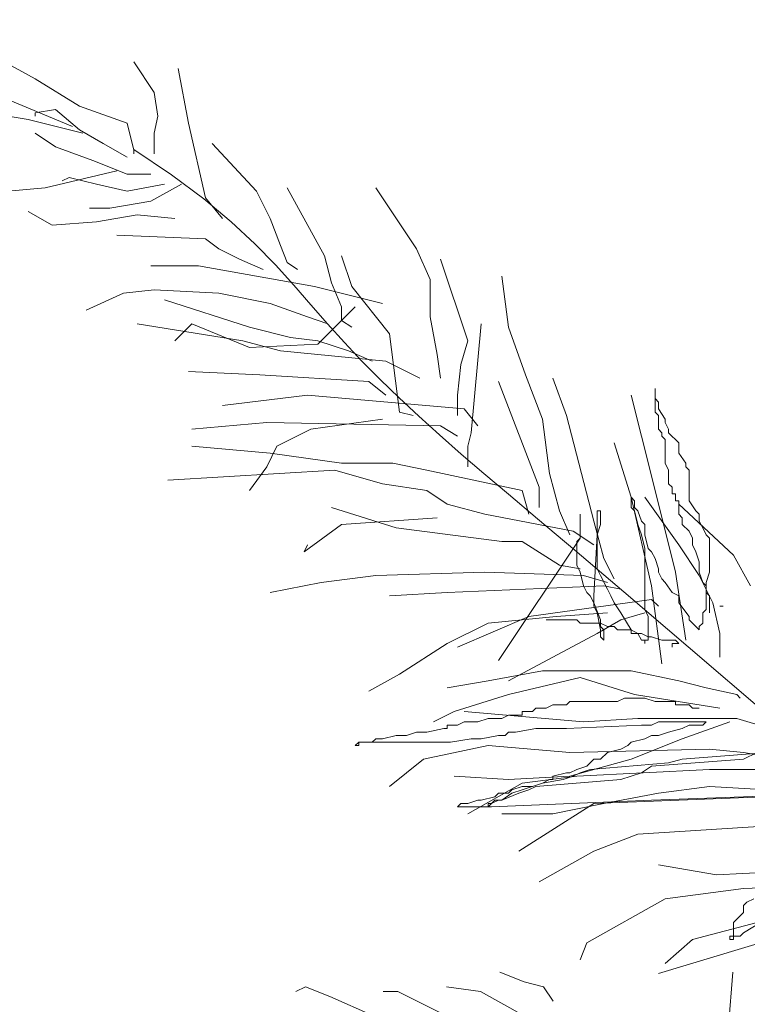
# Model space of a CAD drawing. Units: millimetres. Extents: x 595116 to 630915, y 909473 to 920225.
# Tile 36 of 134: x 629660.182 to 629665.643, y 919173.119 to 919180.516. Entities that reach past the tile are written whole.
import ezdxf

# ---------------------------------------------------------------- set-up
doc = ezdxf.new("R2010")
doc.units = ezdxf.units.MM
doc.layers.add('Dimension', color=3, linetype='Continuous', lineweight=18)
doc.layers.add('L-PLNT', color=85, linetype='Continuous', lineweight=13)
doc.styles.get("Standard").update_dxf_attribs({"font": 'arial.ttf'})
doc.dimstyles.new('ISO-25', dxfattribs={"dimtxt": 9, "dimasz": 6, "dimexe": 1.25, "dimexo": 0.625, "dimtad": 1, "dimlunit": 4, "dimtxsty": 'Standard', "dimcen": 2.5, "dimadec": 0, "dimazin": 0, "dimtfac": 1, "dimtmove": 0, "dimatfit": 3, "dimfxl": 1, "dimarcsym": 0})

# ---------------------------------------------------------------- blocks, each defined once
blk = doc.blocks.new('A$C4FB75ABC')
for p, q in [((0.4999, 4.2779), (0.7111, 4.1621)), ((0.9087, 4.1962), (0.9496, 4.1349)), ((0.9973, 4.1826), (1.0177, 4.0736)), ((0.7111, 4.1621), (0.7997, 4.1076)), ((0.7861, 4.0668), (0.6226, 4.1349)), ((0.9496, 4.1349), (0.9564, 4.0872)), ((0.752, 4.1008), (0.7111, 4.094)), ((0.7997, 4.06), (0.752, 4.1008)), ((0.7997, 4.1076), (0.8951, 4.0736)), ((0.6975, 4.0804), (0.6158, 4.094)), ((0.8065, 4.0532), (0.6975, 4.0804)), ((0.7111, 4.094), (0.7111, 4.0872)), ((0.9564, 4.0872), (0.9496, 4.0532)), ((0.8474, 4.0327), (0.7997, 4.06)), ((0.8951, 4.0736), (0.9087, 4.0191)), ((1.0177, 4.0736), (1.0518, 3.9238)), ((0.7111, 4.0532), (0.752, 4.0259)), ((0.9496, 4.0532), (0.9496, 4.0123)), ((0.752, 4.0259), (0.827, 3.9987)), ((0.8951, 4.0055), (0.8474, 4.0327)), ((0.9842, 3.9699), (0.9085, 4.0207)), ((1.0654, 4.0327), (1.154, 3.9374)), ((0.9087, 4.0191), (0.9087, 4.0123)), ((0.827, 3.9987), (0.8951, 3.9715)), ((0.8746, 3.9783), (0.7316, 3.9442)), ((0.7793, 3.9647), (0.7656, 3.9578)), ((0.8338, 3.951), (0.7793, 3.9647)), ((0.8951, 3.9715), (0.9428, 3.9715)), ((1.0487, 3.9217), (0.9842, 3.9699)), ((0.7316, 3.9442), (0.6566, 3.9374)), ((0.8951, 3.9374), (0.8338, 3.951)), ((0.97, 3.951), (0.8951, 3.9374)), ((1.0041, 3.951), (0.9428, 3.917)), ((1.2153, 3.9442), (1.2902, 3.808)), ((1.3924, 3.9442), (1.4742, 3.8217)), ((1.0518, 3.9238), (1.0858, 3.8829)), ((1.154, 3.9374), (1.1812, 3.8829)), ((0.861, 3.9034), (0.8201, 3.9034)), ((0.9428, 3.917), (0.861, 3.9034)), ((1.1035, 3.8758), (1.0487, 3.9217)), ((0.7452, 3.8693), (0.6975, 3.8966)), ((0.9155, 3.8897), (0.8338, 3.8761)), ((0.9905, 3.8829), (0.9155, 3.8897)), ((1.1812, 3.8829), (1.2017, 3.8285)), ((0.8338, 3.8761), (0.7452, 3.8693)), ((1.1506, 3.8319), (1.1035, 3.8758)), ((0.8746, 3.8489), (1.0518, 3.8421)), ((1.0518, 3.8421), (1.079, 3.8217)), ((1.1917, 3.7897), (1.1506, 3.8319)), ((1.2017, 3.8285), (1.2153, 3.7944)), ((1.079, 3.8217), (1.1199, 3.8012)), ((1.2902, 3.808), (1.3039, 3.7536)), ((1.3243, 3.808), (1.3447, 3.7467)), ((1.4742, 3.8217), (1.5014, 3.7604)), ((0.9428, 3.7876), (1.0382, 3.7876)), ((1.0382, 3.7876), (1.2698, 3.7467)), ((1.1199, 3.8012), (1.1676, 3.7808)), ((1.2284, 3.7492), (1.1917, 3.7897)), ((1.2153, 3.7944), (1.2357, 3.7808)), ((1.5219, 3.8012), (1.5764, 3.6378)), ((1.6445, 3.7672), (1.6581, 3.665)), ((1.2625, 3.7099), (1.2284, 3.7492)), ((1.2698, 3.7467), (1.4061, 3.7127)), ((1.3039, 3.7536), (1.3243, 3.7059)), ((1.3447, 3.7467), (1.4197, 3.6514)), ((1.5014, 3.7604), (1.5014, 3.6855)), ((0.8133, 3.6991), (0.8883, 3.7331)), ((0.8883, 3.7331), (0.9496, 3.7399)), ((0.9496, 3.7399), (1.079, 3.7331)), ((1.079, 3.7331), (1.1812, 3.7127)), ((0.97, 3.7195), (1.1403, 3.665)), ((1.1812, 3.7127), (1.2562, 3.6855)), ((1.2959, 3.6716), (1.2625, 3.7099)), ((1.3515, 3.7059), (1.2766, 3.631)), ((1.3243, 3.7059), (1.3243, 3.6787)), ((1.2562, 3.6855), (1.297, 3.6718)), ((1.5014, 3.6855), (1.5151, 3.6106)), ((0.9155, 3.6718), (1.1267, 3.6378)), ((1.0245, 3.6718), (0.9905, 3.6378)), ((1.1403, 3.6242), (1.0245, 3.6718)), ((1.3299, 3.6341), (1.2959, 3.6716)), ((1.3243, 3.6787), (1.3447, 3.665)), ((1.6036, 3.6718), (1.5832, 3.4539)), ((1.1403, 3.665), (1.2221, 3.6446)), ((1.4197, 3.6514), (1.4401, 3.4948)), ((1.6581, 3.665), (1.6922, 3.5697)), ((1.1267, 3.6378), (1.2017, 3.6174)), ((1.2766, 3.631), (1.1403, 3.6242)), ((1.2221, 3.6446), (1.2766, 3.6378)), ((1.2766, 3.6378), (1.3379, 3.6174)), ((1.365, 3.5971), (1.3299, 3.6341)), ((1.5764, 3.6378), (1.5627, 3.5901)), ((1.2017, 3.6174), (1.4129, 3.5969)), ((1.3379, 3.6174), (1.3856, 3.5969)), ((1.5151, 3.6106), (1.5219, 3.5629)), ((1.4014, 3.5604), (1.365, 3.5971)), ((1.4129, 3.5969), (1.481, 3.5629)), ((1.5627, 3.5901), (1.5559, 3.5288)), ((1.0177, 3.5765), (1.1608, 3.5697)), ((1.1608, 3.5697), (1.3788, 3.5561)), ((1.6922, 3.5697), (1.7263, 3.4812)), ((1.3788, 3.5561), (1.4129, 3.5288)), ((1.4393, 3.5237), (1.4014, 3.5604)), ((1.6377, 3.5561), (1.7194, 3.345)), ((1.7467, 3.5629), (1.7739, 3.488)), ((1.0858, 3.5084), (1.2562, 3.5288)), ((1.2562, 3.5288), (1.5696, 3.5016)), ((1.5559, 3.5288), (1.5559, 3.488)), ((1.9034, 3.5288), (1.9238, 3.4471)), ((1.9511, 3.4948), (1.9511, 3.5425)), ((1.9511, 3.5425), (1.9511, 3.522)), ((1.4788, 3.4868), (1.4393, 3.5237)), ((1.9511, 3.522), (1.9579, 3.5152)), ((1.9579, 3.5152), (1.9579, 3.5016)), ((1.4401, 3.4948), (1.4674, 3.488)), ((1.5696, 3.5016), (1.5968, 3.4676)), ((1.9579, 3.488), (1.9511, 3.4948)), ((1.9579, 3.5016), (1.9715, 3.4812)), ((1.0245, 3.4608), (1.1744, 3.4744)), ((1.1744, 3.4744), (1.5219, 3.4676)), ((1.4061, 3.4812), (1.263, 3.4608)), ((1.5201, 3.4494), (1.4788, 3.4868)), ((1.7263, 3.4812), (1.7399, 3.3722)), ((1.7739, 3.488), (1.8285, 3.2769)), ((1.9579, 3.4608), (1.9579, 3.488)), ((1.9715, 3.4812), (1.9715, 3.4744)), ((1.9715, 3.4744), (1.9783, 3.4608)), ((1.263, 3.4608), (1.1949, 3.4267)), ((1.5633, 3.4112), (1.5201, 3.4494)), ((1.5219, 3.4676), (1.5559, 3.4471)), ((1.5832, 3.4539), (1.5764, 3.4267)), ((1.9647, 3.4539), (1.9579, 3.4608)), ((1.9647, 3.4471), (1.9647, 3.4539)), ((1.9783, 3.4608), (1.9783, 3.4539)), ((1.9783, 3.4539), (1.9988, 3.4335)), ((1.8693, 3.4335), (1.9034, 3.3246)), ((1.9238, 3.4471), (1.9511, 3.3382)), ((1.9715, 3.4403), (1.9647, 3.4471)), ((1.9715, 3.3927), (1.9715, 3.4403)), ((1.9988, 3.4335), (1.9988, 3.4131)), ((1.0245, 3.4267), (1.1812, 3.4131)), ((1.1949, 3.4267), (1.1744, 3.3858)), ((1.1812, 3.4131), (1.3243, 3.3927)), ((1.6088, 3.3721), (1.5633, 3.4112)), ((1.5764, 3.4267), (1.5764, 3.3858)), ((1.9988, 3.4131), (2.0124, 3.3927)), ((1.3243, 3.3927), (1.4265, 3.3927)), ((1.4265, 3.3927), (1.4946, 3.379)), ((1.9783, 3.379), (1.9715, 3.3927)), ((2.0124, 3.3927), (2.0124, 3.3858)), ((0.9768, 3.3586), (1.3107, 3.379)), ((1.1744, 3.3858), (1.1403, 3.3382)), ((1.3107, 3.379), (1.4061, 3.3518)), ((1.4946, 3.379), (1.6854, 3.3382)), ((1.6577, 3.3307), (1.6088, 3.3721)), ((1.7399, 3.3722), (1.7603, 3.2973)), ((1.9783, 3.3518), (1.9783, 3.379)), ((2.0124, 3.3858), (2.0192, 3.379)), ((2.0192, 3.379), (2.0192, 3.3178)), ((1.4061, 3.3518), (1.4946, 3.3382)), ((1.9851, 3.345), (1.9783, 3.3518)), ((1.4946, 3.3382), (1.5355, 3.3109)), ((1.7159, 3.2817), (1.6577, 3.3307)), ((1.6854, 3.3382), (1.699, 3.2905)), ((1.7194, 3.345), (1.7194, 3.3041)), ((1.9511, 3.3382), (1.992, 3.1748)), ((1.9851, 3.3314), (1.9851, 3.345)), ((1.992, 3.3314), (1.9851, 3.3314)), ((1.992, 3.3178), (1.992, 3.3314)), ((1.5355, 3.3109), (1.6104, 3.2905)), ((1.9102, 3.3178), (1.9034, 3.3246)), ((1.9034, 3.3246), (1.9034, 3.3041)), ((1.9034, 3.3246), (1.9443, 3.1475)), ((1.9102, 3.3041), (1.9102, 3.3178)), ((1.9306, 3.3246), (1.9988, 3.2292)), ((1.9988, 3.3178), (1.992, 3.3178)), ((1.9988, 3.2905), (1.9988, 3.3178)), ((1.9988, 3.3109), (2.1078, 3.2088)), ((2.0192, 3.3178), (2.0328, 3.2973)), ((1.3039, 3.3041), (1.4333, 3.2633)), ((1.7603, 3.2973), (1.7808, 3.2497)), ((1.8421, 3.2973), (1.8353, 3.2973)), ((1.8353, 3.2973), (1.8353, 3.2497)), ((1.8421, 3.2701), (1.8421, 3.2973)), ((1.9034, 3.3041), (1.9102, 3.2973)), ((1.917, 3.2973), (1.9102, 3.3041)), ((1.9102, 3.2973), (1.917, 3.2701)), ((1.9238, 3.2769), (1.917, 3.2973)), ((2.0328, 3.2973), (2.0396, 3.2905)), ((1.5151, 3.2837), (1.3243, 3.2701)), ((1.6104, 3.2905), (1.7876, 3.2565)), ((1.7906, 3.2188), (1.7159, 3.2817)), ((1.8012, 3.2429), (1.8012, 3.2905)), ((1.8012, 3.2905), (1.8012, 3.2429)), ((1.8285, 3.2769), (1.8489, 3.202)), ((1.9306, 3.2701), (1.9238, 3.2769)), ((2.0056, 3.2837), (1.9988, 3.2905)), ((2.0056, 3.2701), (2.0056, 3.2837)), ((2.0396, 3.2905), (2.0396, 3.2769)), ((2.0396, 3.2769), (2.0465, 3.2633)), ((1.3243, 3.2701), (1.2494, 3.2156)), ((1.4333, 3.2633), (1.6445, 3.236)), ((1.7876, 3.2565), (1.8285, 3.2292)), ((1.8353, 3.2497), (1.8421, 3.2701)), ((1.917, 3.2701), (1.9238, 3.2497)), ((1.9306, 3.2497), (1.9306, 3.2701)), ((2.0192, 3.2565), (2.0056, 3.2701)), ((2.026, 3.2429), (2.0192, 3.2565)), ((2.0465, 3.2633), (2.0533, 3.2497)), ((1.8012, 3.2429), (1.6377, 2.9977)), ((1.6445, 3.236), (1.6854, 3.236)), ((1.6854, 3.236), (1.7603, 3.1884)), ((1.7944, 3.236), (1.8012, 3.2429)), ((1.7944, 3.1884), (1.7944, 3.236)), ((1.8353, 3.2497), (1.8285, 3.1271)), ((1.8353, 3.1816), (1.8353, 3.2497)), ((1.9238, 3.2497), (1.9306, 3.2224)), ((1.9375, 3.2224), (1.9306, 3.2497)), ((2.026, 3.2292), (2.026, 3.2429)), ((2.0533, 3.2497), (2.0601, 3.2429)), ((2.0601, 3.2429), (2.0601, 3.1748)), ((1.2494, 3.2156), (1.2562, 3.2292)), ((1.8887, 3.1355), (1.7906, 3.2188)), ((1.9306, 3.2224), (1.9306, 3.0999)), ((1.9443, 3.2156), (1.9375, 3.2224)), ((1.9511, 3.202), (1.9443, 3.2156)), ((1.9988, 3.2292), (2.0396, 3.1679)), ((2.0328, 3.2156), (2.026, 3.2292)), ((2.0396, 3.1952), (2.0328, 3.2156)), ((1.8489, 3.202), (1.8693, 3.1611)), ((1.9579, 3.1816), (1.9511, 3.202)), ((2.0396, 3.1748), (2.0396, 3.1952)), ((2.1078, 3.2088), (2.1418, 3.1475)), ((1.3924, 3.1679), (1.6104, 3.1748)), ((1.6104, 3.1748), (1.808, 3.1679)), ((1.7603, 3.1884), (1.8012, 3.1816)), ((1.8012, 3.1748), (1.7944, 3.1884)), ((1.808, 3.1475), (1.8012, 3.1748)), ((1.8421, 3.1679), (1.8353, 3.1816)), ((1.9579, 3.1748), (1.9579, 3.1816)), ((1.9647, 3.1611), (1.9579, 3.1748)), ((1.992, 3.1748), (2.0124, 3.0386)), ((2.0465, 3.1543), (2.0396, 3.1748)), ((2.0601, 3.1748), (2.0533, 3.1543)), ((1.1812, 3.1339), (1.2834, 3.1543)), ((1.2834, 3.1543), (1.3924, 3.1679)), ((1.808, 3.1679), (1.8557, 3.1543)), ((1.8557, 3.1407), (1.8421, 3.1679)), ((1.9715, 3.1543), (1.9647, 3.1611)), ((1.9851, 3.1339), (1.9715, 3.1543)), ((2.0396, 3.1679), (2.0669, 3.1135)), ((2.0533, 3.1475), (2.0465, 3.1543)), ((2.0533, 3.1543), (2.0533, 3.0999)), ((1.4197, 3.1271), (1.5355, 3.1339)), ((1.5355, 3.1339), (1.8489, 3.1475)), ((1.8148, 3.1339), (1.808, 3.1475)), ((1.8216, 3.1271), (1.8148, 3.1339)), ((1.8489, 3.1475), (1.883, 3.1407)), ((1.8625, 3.1271), (1.8557, 3.1407)), ((2.0174, 3.0255), (1.8887, 3.1355)), ((1.9443, 3.1475), (1.9647, 2.9909)), ((1.9988, 3.1271), (1.9851, 3.1339)), ((2.0533, 3.1339), (2.0533, 3.1475)), ((2.0601, 3.1271), (2.0533, 3.1339)), ((1.699, 3.0862), (1.9443, 3.1203)), ((1.8285, 3.1135), (1.8216, 3.1271)), ((1.8285, 3.1271), (1.8285, 3.1067)), ((1.8693, 3.1135), (1.8625, 3.1271)), ((1.9443, 3.1203), (1.9579, 3.1067)), ((1.9988, 3.1135), (1.9988, 3.1271)), ((2.0601, 3.093), (2.0601, 3.1271)), ((1.8421, 3.0794), (1.8285, 3.1135)), ((1.8285, 3.1067), (1.8353, 3.093)), ((1.883, 3.093), (1.8693, 3.1135)), ((1.9306, 3.0999), (1.9375, 3.0862)), ((2.0192, 3.0862), (1.9988, 3.1135)), ((2.0533, 3.0999), (2.0465, 3.093)), ((2.0669, 3.1135), (2.0805, 3.0522)), ((2.0873, 3.1067), (2.0805, 3.1067)), ((1.5559, 3.0249), (1.699, 3.0862)), ((1.7535, 3.0862), (1.6173, 3.0726)), ((1.7331, 3.0794), (1.7944, 3.0794)), ((1.8557, 3.093), (1.7535, 3.0862)), ((1.7944, 3.0794), (1.8012, 3.0726)), ((1.8353, 3.093), (1.8421, 3.059)), ((1.8353, 3.0522), (1.883, 3.0794)), ((1.8421, 3.0658), (1.8421, 3.0794)), ((1.9034, 3.059), (1.883, 3.093)), ((1.883, 3.0794), (1.9306, 3.093)), ((1.9375, 3.0862), (1.9375, 3.0386)), ((2.0192, 3.0794), (2.0192, 3.0862)), ((2.0396, 3.059), (2.0192, 3.0794)), ((2.0465, 3.093), (2.0465, 3.0726)), ((1.6173, 3.0726), (1.5355, 3.0318)), ((1.8012, 3.0726), (1.8421, 3.0726)), ((1.8421, 3.0726), (1.8557, 3.0658)), ((1.8489, 3.059), (1.8421, 3.0658)), ((1.8421, 3.059), (1.8421, 3.0454)), ((1.8489, 3.0386), (1.8489, 3.059)), ((1.8557, 3.0658), (1.8693, 3.0658)), ((1.8693, 3.0658), (1.8761, 3.059)), ((1.8761, 3.059), (1.9034, 3.059)), ((1.917, 3.0522), (1.9034, 3.059)), ((1.9034, 3.059), (1.9034, 3.0522)), ((2.0465, 3.0726), (2.0396, 3.0658)), ((2.0396, 3.0658), (2.0396, 3.059)), ((1.6581, 2.9569), (1.8353, 3.0522)), ((1.8421, 3.0454), (1.8489, 3.0386)), ((1.9034, 3.0522), (1.9238, 3.0522)), ((1.9238, 3.0386), (1.917, 3.0522)), ((1.9238, 3.0522), (1.9375, 3.0454)), ((1.9306, 3.0386), (1.9238, 3.0386)), ((1.9375, 3.0386), (1.9306, 3.0386)), ((1.9306, 3.0386), (1.9306, 3.0318)), ((1.9306, 3.0318), (1.9306, 3.0386)), ((1.9375, 3.0454), (1.9443, 3.0454)), ((1.9443, 3.0454), (1.9647, 3.0386)), ((1.9647, 3.0386), (1.992, 3.0386)), ((1.992, 3.0386), (1.9988, 3.0318)), ((2.0805, 3.0522), (2.0805, 3.0045)), ((1.5355, 3.0318), (1.4401, 2.9705)), ((1.9988, 3.0318), (1.9851, 3.0318)), ((1.9851, 3.0318), (1.9851, 3.0249)), ((2.1835, 2.8826), (2.0174, 3.0255)), ((1.6173, 2.9569), (1.7263, 2.9773)), ((1.7263, 2.9773), (1.9034, 2.9773)), ((1.9034, 2.9773), (1.9988, 2.9569)), ((1.4401, 2.9705), (1.3788, 2.9364)), ((1.5355, 2.9432), (1.6173, 2.9569)), ((1.8012, 2.9637), (1.6581, 2.9296)), ((1.9102, 2.9296), (1.8012, 2.9637)), ((1.9988, 2.9569), (2.0533, 2.9432)), ((2.0533, 2.9432), (2.1146, 2.9296)), ((1.6581, 2.9296), (1.5491, 2.8956)), ((1.8898, 2.9228), (1.8761, 2.916)), ((1.9306, 2.9228), (1.8898, 2.9228)), ((2.0805, 2.9024), (1.9102, 2.9296)), ((1.9511, 2.916), (1.9306, 2.9228)), ((2.1146, 2.9296), (2.1214, 2.9228)), ((1.7126, 2.9024), (1.7058, 2.8956)), ((1.7331, 2.9024), (1.7126, 2.9024)), ((1.7467, 2.9092), (1.7331, 2.9024)), ((1.7739, 2.9092), (1.7467, 2.9092)), ((1.7808, 2.916), (1.7739, 2.9092)), ((1.8761, 2.916), (1.7808, 2.916)), ((1.992, 2.916), (1.9511, 2.916)), ((1.992, 2.9092), (1.992, 2.916)), ((2.0192, 2.9092), (1.992, 2.9092)), ((2.026, 2.9024), (2.0192, 2.9092)), ((2.0396, 2.9024), (2.026, 2.9024)), ((1.5491, 2.8956), (1.5082, 2.8751)), ((1.5696, 2.8956), (1.808, 2.8751)), ((1.6173, 2.882), (1.5968, 2.8751)), ((1.6445, 2.882), (1.6173, 2.882)), ((1.6581, 2.8888), (1.6445, 2.882)), ((1.6854, 2.8888), (1.6581, 2.8888)), ((1.6854, 2.8956), (1.6854, 2.8888)), ((1.7058, 2.8956), (1.6854, 2.8956)), ((1.808, 2.8751), (1.917, 2.882)), ((1.917, 2.882), (2.1146, 2.882)), ((2.1146, 2.882), (2.1827, 2.8615)), ((1.5287, 2.8615), (1.4946, 2.8547)), ((1.5355, 2.8615), (1.5287, 2.8615)), ((1.5559, 2.8683), (1.5355, 2.8683)), ((1.5355, 2.8683), (1.5355, 2.8615)), ((1.5696, 2.8751), (1.5559, 2.8683)), ((1.5968, 2.8751), (1.5696, 2.8751)), ((1.6718, 2.8547), (1.7126, 2.8615)), ((1.7126, 2.8615), (1.7739, 2.8615)), ((1.7739, 2.8615), (1.9238, 2.8683)), ((1.9238, 2.8683), (1.9443, 2.8683)), ((1.9443, 2.8683), (1.9579, 2.8751)), ((1.9579, 2.8751), (2.0533, 2.8751)), ((2.0056, 2.8615), (1.9783, 2.8547)), ((2.101, 2.8751), (2.0056, 2.8411)), ((2.0192, 2.8683), (2.0056, 2.8615)), ((2.0465, 2.8683), (2.0192, 2.8683)), ((2.0533, 2.8751), (2.0465, 2.8683)), ((1.3924, 2.8411), (1.3856, 2.8343)), ((1.4061, 2.8411), (1.3924, 2.8411)), ((1.4333, 2.8479), (1.4061, 2.8411)), ((1.4537, 2.8479), (1.4333, 2.8479)), ((1.4742, 2.8547), (1.4537, 2.8479)), ((1.4946, 2.8547), (1.4742, 2.8547)), ((1.5423, 2.8343), (1.5832, 2.8411)), ((1.5832, 2.8411), (1.6036, 2.8411)), ((1.6036, 2.8411), (1.6377, 2.8479)), ((1.6377, 2.8479), (1.6513, 2.8479)), ((1.6513, 2.8479), (1.6581, 2.8547)), ((1.6581, 2.8547), (1.6718, 2.8547)), ((1.9306, 2.8411), (1.9034, 2.8343)), ((2.0056, 2.8411), (1.9034, 2.8002)), ((1.9443, 2.8479), (1.9306, 2.8411)), ((1.9579, 2.8479), (1.9443, 2.8479)), ((1.9783, 2.8547), (1.9579, 2.8479)), ((1.3515, 2.8275), (1.3584, 2.8343)), ((1.3584, 2.8275), (1.3515, 2.8275)), ((1.3856, 2.8343), (1.3584, 2.8343)), ((1.3584, 2.8343), (1.3584, 2.8275)), ((1.3584, 2.8343), (1.5423, 2.8343)), ((1.4878, 2.8002), (1.6173, 2.8275)), ((1.6173, 2.8275), (1.7808, 2.8139)), ((1.7808, 2.8139), (2.0601, 2.8207)), ((1.883, 2.8207), (1.8557, 2.8139)), ((1.8966, 2.8275), (1.883, 2.8207)), ((1.9034, 2.8343), (1.8966, 2.8275)), ((2.0601, 2.8207), (2.1282, 2.8139)), ((1.4197, 2.7458), (1.4878, 2.8002)), ((1.9034, 2.8002), (1.7808, 2.7662)), ((1.8285, 2.8002), (1.8148, 2.7866)), ((1.8421, 2.8002), (1.8285, 2.8002)), ((1.8557, 2.8139), (1.8421, 2.8002)), ((1.9443, 2.7866), (2.1282, 2.8002)), ((2.0056, 2.8002), (1.9783, 2.7934)), ((2.1759, 2.8139), (2.0056, 2.8002)), ((2.1282, 2.8002), (2.1555, 2.8139)), ((2.1282, 2.8139), (2.2917, 2.7866)), ((1.7944, 2.7798), (1.7808, 2.773)), ((1.8148, 2.7866), (1.7944, 2.7798)), ((1.7944, 2.7662), (2.0601, 2.7798)), ((1.8216, 2.7798), (1.8012, 2.773)), ((1.9783, 2.7934), (1.8216, 2.7798)), ((1.9238, 2.773), (1.9443, 2.7866)), ((2.0601, 2.7798), (2.1078, 2.7798)), ((2.1078, 2.7798), (2.1963, 2.7798)), ((1.6581, 2.7594), (1.5491, 2.7662)), ((1.7808, 2.7662), (1.6581, 2.7594)), ((1.6854, 2.7526), (1.7944, 2.7662)), ((1.7126, 2.7458), (1.883, 2.7594)), ((1.7399, 2.7594), (1.7263, 2.7526)), ((1.7671, 2.7594), (1.7263, 2.7526)), ((1.7467, 2.7594), (1.7399, 2.7594)), ((1.7739, 2.773), (1.7467, 2.7662)), ((1.7467, 2.7662), (1.7467, 2.7594)), ((1.7876, 2.7662), (1.7671, 2.7594)), ((1.7808, 2.773), (1.7739, 2.773)), ((1.8012, 2.773), (1.7876, 2.7662)), ((1.883, 2.7594), (1.9034, 2.7662)), ((1.9034, 2.7662), (1.9238, 2.773)), ((1.5764, 2.6913), (1.6854, 2.7526)), ((1.6854, 2.7458), (1.6649, 2.739)), ((1.7263, 2.7526), (1.6854, 2.739)), ((1.7058, 2.7458), (1.6854, 2.7458)), ((1.699, 2.739), (1.7126, 2.7458)), ((1.7263, 2.7526), (1.7058, 2.7458)), ((2.0601, 2.7458), (1.9579, 2.7321)), ((2.1759, 2.739), (2.0601, 2.7458)), ((1.6309, 2.7253), (1.6036, 2.7185)), ((1.6377, 2.7321), (1.6309, 2.7253)), ((1.6581, 2.7321), (1.6377, 2.7321)), ((1.6649, 2.7321), (1.6445, 2.7185)), ((1.6445, 2.7185), (1.6786, 2.7321)), ((1.6649, 2.739), (1.6581, 2.7321)), ((1.6854, 2.739), (1.6649, 2.7321)), ((1.6786, 2.7321), (1.699, 2.739)), ((1.8285, 2.7117), (2.1691, 2.7253)), ((1.9579, 2.7321), (1.8489, 2.7117)), ((1.9443, 2.7185), (2.1282, 2.7253)), ((2.1282, 2.7253), (2.3122, 2.7321)), ((1.5627, 2.7117), (1.5559, 2.7049)), ((1.5559, 2.7049), (1.6241, 2.7049)), ((1.5764, 2.7117), (1.5627, 2.7117)), ((1.5968, 2.7185), (1.5764, 2.7117)), ((1.6036, 2.7185), (1.5968, 2.7185)), ((1.6309, 2.7185), (1.6173, 2.7049)), ((1.6173, 2.7049), (1.6173, 2.7117)), ((1.6173, 2.7117), (1.6241, 2.7117)), ((1.6241, 2.7117), (1.6377, 2.7185)), ((1.6241, 2.7049), (1.9443, 2.7185)), ((1.6445, 2.7185), (1.6309, 2.7185)), ((1.6377, 2.7185), (1.6445, 2.7185)), ((1.6786, 2.6164), (1.8285, 2.7117)), ((1.8489, 2.7117), (1.7467, 2.6913)), ((1.7467, 2.6913), (1.6445, 2.6913)), ((1.917, 2.6504), (2.2372, 2.6709)), ((1.8285, 2.6164), (1.917, 2.6504)), ((1.7194, 2.5551), (1.8285, 2.6164)), ((2.0737, 2.5687), (1.9579, 2.5891)), ((2.2032, 2.5755), (2.0737, 2.5687)), ((2.5234, 2.5551), (2.1282, 2.5415)), ((2.1282, 2.5415), (1.9715, 2.5211)), ((1.9715, 2.5211), (1.8148, 2.4325)), ((2.135, 2.5142), (2.1282, 2.5074)), ((2.1282, 2.5074), (2.1282, 2.4938)), ((2.1487, 2.5211), (2.135, 2.5142)), ((2.1282, 2.4938), (2.1146, 2.4802)), ((2.1555, 2.4734), (2.026, 2.4393)), ((2.1146, 2.4802), (2.1078, 2.4734)), ((2.1078, 2.4734), (2.1078, 2.4461)), ((2.1282, 2.453), (2.1623, 2.4734)), ((2.1078, 2.4461), (2.101, 2.4461)), ((2.101, 2.4461), (2.101, 2.4393)), ((2.1078, 2.4393), (2.1078, 2.4461)), ((2.1078, 2.4461), (2.1214, 2.4461)), ((2.1214, 2.4461), (2.1282, 2.453)), ((1.8148, 2.4325), (1.8012, 2.3985)), ((2.1827, 2.4393), (1.9579, 2.3712)), ((2.026, 2.4393), (1.9715, 2.3917)), ((2.101, 2.4393), (2.1078, 2.4393)), ((1.6891, 2.3546), (1.6405, 2.3741)), ((2.1065, 2.3741), (2.087, 2.1315)), ((1.7279, 2.3449), (1.6891, 2.3546)), ((1.2522, 2.3449), (1.2328, 2.3352)), ((1.3008, 2.3255), (1.2522, 2.3449)), ((1.3881, 2.2867), (1.3008, 2.3255)), ((1.4367, 2.3352), (1.4075, 2.3352)), ((1.5337, 2.2867), (1.4367, 2.3352)), ((1.6017, 2.3352), (1.5337, 2.3449)), ((1.6891, 2.2867), (1.6017, 2.3352)), ((1.7473, 2.3158), (1.7279, 2.3449))]:
    blk.add_line(p, q)
blk = doc.blocks.new('*D216')
at = {"layer": 'Defpoints', "color": 0, "transparency": 16777216}
for p in [(629743.5408, 919411.9276), (629505.0408, 919411.8279), (629743.5408, 918832.3776)]:
    blk.add_point(p, dxfattribs=at)
at = {"layer": 'Dimension', "color": 0, "lineweight": -2, "transparency": 16777216}
for p, q in [((629743.5408, 919411.3026), (629743.5408, 918831.1276)), ((629505.0408, 919411.2029), (629505.0408, 918831.1276)), ((629511.0408, 918832.3776), (629737.5408, 918832.3776))]:
    blk.add_line(p, q, dxfattribs=at)
at = {"layer": 'Dimension', "color": 0, "transparency": 16777216}
for points in [[(629511.0408, 918833.3776), (629511.0408, 918831.3776), (629505.0408, 918832.3776)], [(629737.5408, 918833.3776), (629737.5408, 918831.3776), (629743.5408, 918832.3776)]]:
    blk.add_solid(points, dxfattribs=at)
at = {"layer": 'Dimension', "color": 0, "transparency": 16777216, "insert": (629624.2908, 918837.656), "char_height": 9, "attachment_point": 5}
blk.add_mtext('19\'-10 1/2"', dxfattribs=at)

msp = doc.modelspace()

# ---------------------------------------------------------------- block references
at = {"layer": 'L-PLNT', "xscale": 3.753413438031968, "yscale": 3.753413438031968, "zscale": 3.753413438031968}
msp.add_blockref('A$C4FB75ABC', (629657.6275, 919164.4492), dxfattribs=at)

# ---------------------------------------------------------------- dimensions: what is measured, and where the dimension line sits
at = {"layer": 'Dimension'}
dim = msp.add_linear_dim(base=(629743.5408, 918832.3776), p1=(629505.0408, 919411.8279), p2=(629743.5408, 919411.9276), dimstyle='ISO-25', override={"dimdec": 1, "dimlfac": 1, "dimrnd": 0, "dimzin": 1, "dimdsep": 46, "dimlunit": 4, "dimfrac": 2}, dxfattribs=at)
dim.commit()
dim.dimension.update_dxf_attribs({"geometry": '*D216', "text_midpoint": (629624.2908, 918837.656)})

doc.saveas('drawing.dxf')
